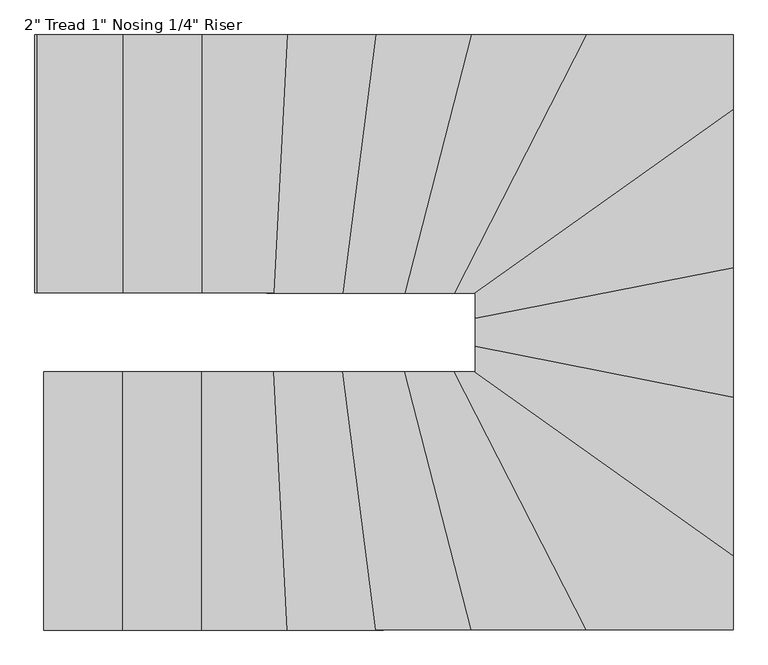
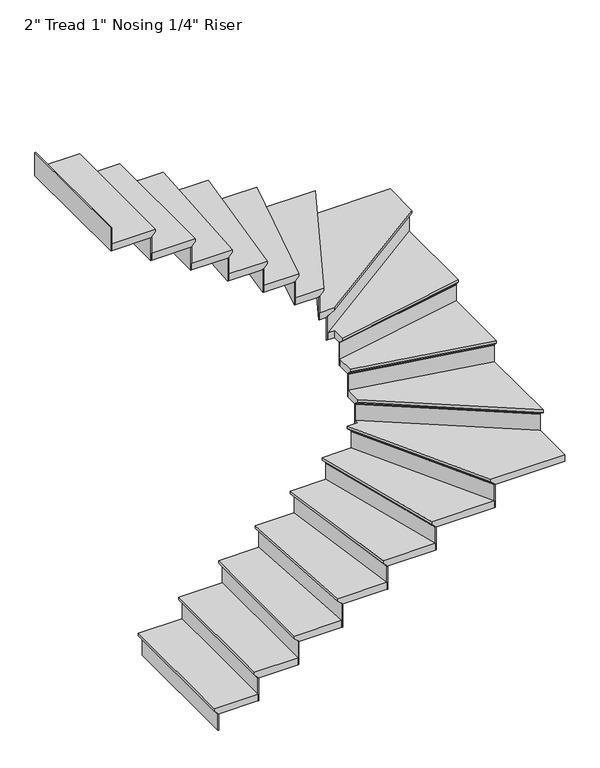
"""IFC4 building model written with IfcOpenShell, lengths in millimetres: stair flight geometry."""

from ifc_helpers import new_model, si_unit, origin, place, context, project, spatial, faceted_brep, source, transform, mapped, element, save


def stair_flight_09daeeff(model_context):
    return source(origin(), model_context, "Body", "Brep", [
        faceted_brep([(531.7538115, -7565.2090409, 16152.2833333), (531.7538115, -7565.2090409, 16171.3333333), (531.7538115, -6650.8090409, 16171.3333333), (531.7538115, -6650.8090409, 16152.2833333), (557.1538115, -7565.2090409, 16126.8833333), (557.1538115, -6650.8090409, 16126.8833333), (836.5538115, -7565.2090409, 16171.3333333), (836.5538115, -6650.8090409, 16171.3333333), (557.1538115, -6650.8090409, 16120.5333333), (836.5538115, -6650.8090409, 16120.5333333), (836.5538115, -7565.2090409, 16120.5333333), (557.1538115, -7565.2090409, 16120.5333333)], [[[0, 1, 2, 3]], [[4, 0, 3, 5]], [[2, 1, 6, 7]], [[8, 9, 10, 11]], [[2, 7, 9, 8, 5, 3]], [[8, 11, 4, 5]], [[6, 1, 0, 4, 11, 10]], [[7, 6, 10, 9]]]),
        faceted_brep([(557.1538115, -7565.2090409, 16120.5333333), (557.1538115, -7565.2090409, 16002.0), (563.5038115, -7565.2090409, 16002.0), (563.5038115, -7565.2090409, 16120.5333333), (557.1538115, -6650.8090409, 16120.5333333), (563.5038115, -6650.8090409, 16120.5333333), (563.5038115, -6650.8090409, 16002.0), (557.1538115, -6650.8090409, 16002.0)], [[[0, 1, 2, 3]], [[4, 5, 6, 7]], [[1, 0, 4, 7]], [[2, 1, 7, 6]], [[3, 2, 6, 5]], [[0, 3, 5, 4]]]),
        faceted_brep([(836.5538115, -7565.2090409, 16289.8666667), (836.5538115, -7565.2090409, 16120.5333333), (842.9038115, -7565.2090409, 16120.5333333), (842.9038115, -7565.2090409, 16289.8666667), (836.5538115, -6650.8090409, 16289.8666667), (842.9038115, -6650.8090409, 16289.8666667), (842.9038115, -6650.8090409, 16120.5333333), (836.5538115, -6650.8090409, 16120.5333333)], [[[0, 1, 2, 3]], [[4, 5, 6, 7]], [[1, 0, 4, 7]], [[2, 1, 7, 6]], [[3, 2, 6, 5]], [[0, 3, 5, 4]]]),
        faceted_brep([(811.1538115, -6650.8090409, 16340.6666667), (811.1538115, -7565.2090409, 16340.6666667), (1115.9538115, -7565.2090409, 16340.6666667), (1115.9538115, -6650.8090409, 16340.6666667), (836.5538115, -6650.8090409, 16289.8666667), (1115.9538115, -6650.8090409, 16289.8666667), (1115.9538115, -7565.2090409, 16289.8666667), (836.5538115, -7565.2090409, 16289.8666667), (836.5538115, -6650.8090409, 16296.2166667), (811.1538115, -6650.8090409, 16321.6166667), (836.5538115, -7565.2090409, 16296.2166667), (811.1538115, -7565.2090409, 16321.6166667)], [[[0, 1, 2, 3]], [[4, 5, 6, 7]], [[0, 3, 5, 4, 8, 9]], [[4, 7, 10, 8]], [[2, 1, 11, 10, 7, 6]], [[3, 2, 6, 5]], [[11, 1, 0, 9]], [[10, 11, 9, 8]]]),
        faceted_brep([(1115.9538115, -7565.2090409, 16459.2), (1115.9538115, -7565.2090409, 16289.8666667), (1122.3038115, -7565.2090409, 16289.8666667), (1122.3038115, -7565.2090409, 16459.2), (1115.9538115, -6650.8090409, 16459.2), (1122.3038115, -6650.8090409, 16459.2), (1122.3038115, -6650.8090409, 16289.8666667), (1115.9538115, -6650.8090409, 16289.8666667)], [[[0, 1, 2, 3]], [[4, 5, 6, 7]], [[1, 0, 4, 7]], [[2, 1, 7, 6]], [[3, 2, 6, 5]], [[0, 3, 5, 4]]]),
        faceted_brep([(1090.5538115, -6650.8090409, 16510.0), (1090.5538115, -7565.2090409, 16510.0), (1419.1552434, -7565.2090409, 16510.0), (1371.620973, -6650.8090409, 16510.0), (1115.9538115, -6650.8090409, 16459.2), (1371.620973, -6650.8090409, 16459.2), (1419.1552434, -7565.2090409, 16459.2), (1115.9538115, -7565.2090409, 16459.2), (1115.9538115, -6650.8090409, 16465.55), (1090.5538115, -6650.8090409, 16490.95), (1115.9538115, -7565.2090409, 16465.55), (1090.5538115, -7565.2090409, 16490.95)], [[[0, 1, 2, 3]], [[4, 5, 6, 7]], [[0, 3, 5, 4, 8, 9]], [[4, 7, 10, 8]], [[2, 1, 11, 10, 7, 6]], [[3, 2, 6, 5]], [[11, 1, 0, 9]], [[10, 11, 9, 8]]]),
        faceted_brep([(1419.1552434, -7565.2090409, 16628.5333333), (1419.1552434, -7565.2090409, 16459.2), (1425.5138176, -7565.2090409, 16459.2), (1425.5138176, -7565.2090409, 16628.5333333), (1371.620973, -6650.8090409, 16628.5333333), (1377.9795471, -6650.8090409, 16628.5333333), (1377.9795471, -6650.8090409, 16459.2), (1371.620973, -6650.8090409, 16459.2)], [[[0, 1, 2, 3]], [[4, 5, 6, 7]], [[1, 0, 4, 7]], [[2, 1, 7, 6]], [[3, 2, 6, 5]], [[0, 3, 5, 4]]]),
        faceted_brep([(1346.1866763, -6650.8090409, 16679.3333333), (1393.7209467, -7565.2090409, 16679.3333333), (1734.1437245, -7565.2090409, 16679.3333333), (1615.7876728, -6650.8090409, 16679.3333333), (1371.620973, -6650.8090409, 16628.5333333), (1615.7876728, -6650.8090409, 16628.5333333), (1734.1437245, -7565.2090409, 16628.5333333), (1419.1552434, -7565.2090409, 16628.5333333), (1371.620973, -6650.8090409, 16634.8833333), (1346.1866763, -6650.8090409, 16660.2833333), (1419.1552434, -7565.2090409, 16634.8833333), (1393.7209467, -7565.2090409, 16660.2833333)], [[[0, 1, 2, 3]], [[4, 5, 6, 7]], [[0, 3, 5, 4, 8, 9]], [[4, 7, 10, 8]], [[2, 1, 11, 10, 7, 6]], [[3, 2, 6, 5]], [[11, 1, 0, 9]], [[10, 11, 9, 8]]]),
        faceted_brep([(1734.1437245, -7565.2090409, 16797.8666667), (1734.1437245, -7565.2090409, 16628.5333333), (1740.5466962, -7565.2090409, 16628.5333333), (1740.5466962, -7565.2090409, 16797.8666667), (1615.7876728, -6650.8090409, 16797.8666667), (1622.1906446, -6650.8090409, 16797.8666667), (1622.1906446, -6650.8090409, 16628.5333333), (1615.7876728, -6650.8090409, 16628.5333333)], [[[0, 1, 2, 3]], [[4, 5, 6, 7]], [[1, 0, 4, 7]], [[2, 1, 7, 6]], [[3, 2, 6, 5]], [[0, 3, 5, 4]]]),
        faceted_brep([(1590.1757857, -6650.8090409, 16848.6666667), (1708.5318374, -7565.2090409, 16848.6666667), (2072.5453427, -7565.2090409, 16848.6666667), (1837.4148953, -6650.8090409, 16848.6666667), (1615.7876728, -6650.8090409, 16797.8666667), (1837.4148953, -6650.8090409, 16797.8666667), (2072.5453427, -7565.2090409, 16797.8666667), (1734.1437245, -7565.2090409, 16797.8666667), (1615.7876728, -6650.8090409, 16804.2166667), (1590.1757857, -6650.8090409, 16829.6166667), (1734.1437245, -7565.2090409, 16804.2166667), (1708.5318374, -7565.2090409, 16829.6166667)], [[[0, 1, 2, 3]], [[4, 5, 6, 7]], [[0, 3, 5, 4, 8, 9]], [[4, 7, 10, 8]], [[2, 1, 11, 10, 7, 6]], [[3, 2, 6, 5]], [[11, 1, 0, 9]], [[10, 11, 9, 8]]]),
        faceted_brep([(2072.5453427, -7565.2090409, 16967.2), (2072.5453427, -7565.2090409, 16797.8666667), (2079.1019196, -7565.2090409, 16797.8666667), (2079.1019196, -7565.2090409, 16967.2), (1837.4148953, -6650.8090409, 16967.2), (1843.9714722, -6650.8090409, 16967.2), (1843.9714722, -6650.8090409, 16797.8666667), (1837.4148953, -6650.8090409, 16797.8666667)], [[[0, 1, 2, 3]], [[4, 5, 6, 7]], [[1, 0, 4, 7]], [[2, 1, 7, 6]], [[3, 2, 6, 5]], [[0, 3, 5, 4]]]),
        faceted_brep([(1811.1885878, -6650.8090409, 17018.0), (2046.3190352, -7565.2090409, 17018.0), (2482.5861527, -7565.2090409, 17018.0), (2013.7615314, -6650.8090409, 17018.0), (1837.4148953, -6650.8090409, 16967.2), (2013.7615314, -6650.8090409, 16967.2), (2482.5861527, -7565.2090409, 16967.2), (2072.5453427, -7565.2090409, 16967.2), (1837.4148953, -6650.8090409, 16973.55), (1811.1885878, -6650.8090409, 16998.95), (2072.5453427, -7565.2090409, 16973.55), (2046.3190352, -7565.2090409, 16998.95)], [[[0, 1, 2, 3]], [[4, 5, 6, 7]], [[0, 3, 5, 4, 8, 9]], [[4, 7, 10, 8]], [[2, 1, 11, 10, 7, 6]], [[3, 2, 6, 5]], [[11, 1, 0, 9]], [[10, 11, 9, 8]]]),
        faceted_brep([(2482.5861527, -7565.2090409, 17136.5333333), (2482.5861527, -7565.2090409, 16967.2), (2489.7221358, -7565.2090409, 16967.2), (2489.7221358, -7565.2090409, 17136.5333333), (2013.7615314, -6650.8090409, 17136.5333333), (2020.8975145, -6650.8090409, 17136.5333333), (2020.8975145, -6650.8090409, 16967.2), (2013.7615314, -6650.8090409, 16967.2)], [[[0, 1, 2, 3]], [[4, 5, 6, 7]], [[1, 0, 4, 7]], [[2, 1, 7, 6]], [[3, 2, 6, 5]], [[0, 3, 5, 4]]]),
        faceted_brep([(2059.4855034, -6621.253958, 17187.3333333), (2059.4855034, -6650.8090409, 17187.3333333), (1985.2175988, -6650.8090409, 17187.3333333), (2454.0422202, -7565.2090409, 17187.3333333), (2973.8855034, -7565.2090409, 17187.3333333), (2973.8855034, -7271.5279072, 17187.3333333), (2059.4855034, -6650.8090409, 17136.5333333), (2059.4855034, -6621.253958, 17136.5333333), (2973.8855034, -7271.5279072, 17136.5333333), (2973.8855034, -7565.2090409, 17136.5333333), (2482.5861527, -7565.2090409, 17136.5333333), (2013.7615314, -6650.8090409, 17136.5333333), (2013.7615314, -6650.8090409, 17142.8833333), (1985.2175988, -6650.8090409, 17168.2833333), (2482.5861527, -7565.2090409, 17142.8833333), (2454.0422202, -7565.2090409, 17168.2833333)], [[[0, 1, 2, 3, 4, 5]], [[6, 7, 8, 9, 10, 11]], [[1, 0, 7, 6]], [[2, 1, 6, 11, 12, 13]], [[11, 10, 14, 12]], [[4, 3, 15, 14, 10, 9]], [[5, 4, 9, 8]], [[0, 5, 8, 7]], [[15, 3, 2, 13]], [[14, 15, 13, 12]]]),
        faceted_brep([(2973.8855034, -7271.5279072, 17305.8666667), (2973.8855034, -7271.5279072, 17136.5333333), (2973.8855034, -7263.7359324, 17136.5333333), (2973.8855034, -7263.7359324, 17305.8666667), (2059.4855034, -6621.253958, 17305.8666667), (2059.4855034, -6613.4619832, 17305.8666667), (2059.4855034, -6613.4619832, 17136.5333333), (2059.4855034, -6621.253958, 17136.5333333)], [[[0, 1, 2, 3]], [[4, 5, 6, 7]], [[1, 0, 4, 7]], [[2, 1, 7, 6]], [[3, 2, 6, 5]], [[0, 3, 5, 4]]]),
        faceted_brep([(2059.4855034, -6652.4218572, 17356.6666667), (2973.8855034, -7302.6958063, 17356.6666667), (2973.8855034, -6715.0407273, 17356.6666667), (2059.4855034, -6534.7998709, 17356.6666667), (2059.4855034, -6621.253958, 17305.8666667), (2059.4855034, -6534.7998709, 17305.8666667), (2973.8855034, -6715.0407273, 17305.8666667), (2973.8855034, -7271.5279072, 17305.8666667), (2059.4855034, -6621.253958, 17312.2166667), (2059.4855034, -6652.4218572, 17337.6166667), (2973.8855034, -7271.5279072, 17312.2166667), (2973.8855034, -7302.6958063, 17337.6166667)], [[[0, 1, 2, 3]], [[4, 5, 6, 7]], [[0, 3, 5, 4, 8, 9]], [[4, 7, 10, 8]], [[3, 2, 6, 5]], [[11, 1, 0, 9]], [[10, 11, 9, 8]], [[2, 1, 11, 10, 7, 6]]]),
        faceted_brep([(2973.8855034, -6715.0407273, 17475.2), (2973.8855034, -6715.0407273, 17305.8666667), (2973.8855034, -6708.5685418, 17305.8666667), (2973.8855034, -6708.5685418, 17475.2), (2059.4855034, -6534.7998709, 17475.2), (2059.4855034, -6528.3276855, 17475.2), (2059.4855034, -6528.3276855, 17305.8666667), (2059.4855034, -6534.7998709, 17305.8666667)], [[[0, 1, 2, 3]], [[4, 5, 6, 7]], [[1, 0, 4, 7]], [[2, 1, 7, 6]], [[3, 2, 6, 5]], [[0, 3, 5, 4]]]),
        faceted_brep([(2059.4855034, -6560.6886127, 17526.0), (2973.8855034, -6740.929469, 17526.0), (2973.8855034, -6255.3998709, 17526.0), (2059.4855034, -6435.6407273, 17526.0), (2059.4855034, -6534.7998709, 17475.2), (2059.4855034, -6435.6407273, 17475.2), (2973.8855034, -6255.3998709, 17475.2), (2973.8855034, -6715.0407273, 17475.2), (2059.4855034, -6534.7998709, 17481.55), (2059.4855034, -6560.6886127, 17506.95), (2973.8855034, -6715.0407273, 17481.55), (2973.8855034, -6740.929469, 17506.95)], [[[0, 1, 2, 3]], [[4, 5, 6, 7]], [[0, 3, 5, 4, 8, 9]], [[4, 7, 10, 8]], [[2, 1, 11, 10, 7, 6]], [[3, 2, 6, 5]], [[11, 1, 0, 9]], [[10, 11, 9, 8]]]),
        faceted_brep([(2973.8855034, -6255.3998709, 17644.5333333), (2973.8855034, -6255.3998709, 17475.2), (2973.8855034, -6248.9276855, 17475.2), (2973.8855034, -6248.9276855, 17644.5333333), (2059.4855034, -6435.6407273, 17644.5333333), (2059.4855034, -6429.1685418, 17644.5333333), (2059.4855034, -6429.1685418, 17475.2), (2059.4855034, -6435.6407273, 17475.2)], [[[0, 1, 2, 3]], [[4, 5, 6, 7]], [[1, 0, 4, 7]], [[2, 1, 7, 6]], [[3, 2, 6, 5]], [[0, 3, 5, 4]]]),
        faceted_brep([(2013.3900289, -6371.4090409, 17695.3333333), (2059.4855034, -6371.4090409, 17695.3333333), (2059.4855034, -6461.529469, 17695.3333333), (2973.8855034, -6281.2886127, 17695.3333333), (2973.8855034, -5688.3543762, 17695.3333333), (2059.4855034, -6371.4090409, 17644.5333333), (2013.3900289, -6371.4090409, 17644.5333333), (2973.8855034, -5688.3543762, 17644.5333333), (2973.8855034, -6255.3998709, 17644.5333333), (2059.4855034, -6435.6407273, 17644.5333333), (2973.8855034, -6255.3998709, 17650.8833333), (2059.4855034, -6435.6407273, 17650.8833333), (2973.8855034, -6281.2886127, 17676.2833333), (2059.4855034, -6461.529469, 17676.2833333)], [[[0, 1, 2, 3, 4]], [[5, 6, 7, 8, 9]], [[1, 0, 6, 5]], [[9, 8, 10, 11]], [[4, 3, 12, 10, 8, 7]], [[0, 4, 7, 6]], [[12, 3, 2, 13]], [[10, 12, 13, 11]], [[2, 1, 5, 9, 11, 13]]]),
        faceted_brep([(2973.8855034, -5688.3543762, 17813.8666667), (2973.8855034, -5688.3543762, 17644.5333333), (2973.8855034, -5680.5624014, 17644.5333333), (2973.8855034, -5680.5624014, 17813.8666667), (2013.3900289, -6371.4090409, 17813.8666667), (2002.4331364, -6371.4090409, 17813.8666667), (2002.4331364, -6371.4090409, 17644.5333333), (2013.3900289, -6371.4090409, 17644.5333333)], [[[0, 1, 2, 3]], [[4, 5, 6, 7]], [[1, 0, 4, 7]], [[2, 1, 7, 6]], [[3, 2, 6, 5]], [[0, 3, 5, 4]]]),
        faceted_brep([(2057.2175988, -6371.4090409, 17864.6666667), (2973.8855034, -5719.5222754, 17864.6666667), (2973.8855034, -5457.0090409, 17864.6666667), (2425.4982876, -5457.0090409, 17864.6666667), (1956.6736663, -6371.4090409, 17864.6666667), (2013.3900289, -6371.4090409, 17813.8666667), (1956.6736663, -6371.4090409, 17813.8666667), (2425.4982876, -5457.0090409, 17813.8666667), (2973.8855034, -5457.0090409, 17813.8666667), (2973.8855034, -5688.3543762, 17813.8666667), (2013.3900289, -6371.4090409, 17820.2166667), (2057.2175988, -6371.4090409, 17845.6166667), (2973.8855034, -5688.3543762, 17820.2166667), (2973.8855034, -5719.5222754, 17845.6166667)], [[[0, 1, 2, 3, 4]], [[5, 6, 7, 8, 9]], [[0, 4, 6, 5, 10, 11]], [[5, 9, 12, 10]], [[2, 1, 13, 12, 9, 8]], [[4, 3, 7, 6]], [[13, 1, 0, 11]], [[12, 13, 11, 10]], [[3, 2, 8, 7]]]),
        faceted_brep([(2425.4982876, -5457.0090409, 17983.2), (2425.4982876, -5457.0090409, 17813.8666667), (2418.3623045, -5457.0090409, 17813.8666667), (2418.3623045, -5457.0090409, 17983.2), (1956.6736663, -6371.4090409, 17983.2), (1949.5376832, -6371.4090409, 17983.2), (1949.5376832, -6371.4090409, 17813.8666667), (1956.6736663, -6371.4090409, 17813.8666667)], [[[0, 1, 2, 3]], [[4, 5, 6, 7]], [[1, 0, 4, 7]], [[2, 1, 7, 6]], [[3, 2, 6, 5]], [[0, 3, 5, 4]]]),
        faceted_brep([(1985.2175988, -6371.4090409, 18034.0), (2454.0422202, -5457.0090409, 18034.0), (2020.0927278, -5457.0090409, 18034.0), (1784.9622804, -6371.4090409, 18034.0), (1956.6736663, -6371.4090409, 17983.2), (1784.9622804, -6371.4090409, 17983.2), (2020.0927278, -5457.0090409, 17983.2), (2425.4982876, -5457.0090409, 17983.2), (1956.6736663, -6371.4090409, 17989.55), (1985.2175988, -6371.4090409, 18014.95), (2425.4982876, -5457.0090409, 17989.55), (2454.0422202, -5457.0090409, 18014.95)], [[[0, 1, 2, 3]], [[4, 5, 6, 7]], [[0, 3, 5, 4, 8, 9]], [[4, 7, 10, 8]], [[2, 1, 11, 10, 7, 6]], [[3, 2, 6, 5]], [[11, 1, 0, 9]], [[10, 11, 9, 8]]]),
        faceted_brep([(2020.0927278, -5457.0090409, 18152.5333333), (2020.0927278, -5457.0090409, 17983.2), (2013.5361509, -5457.0090409, 17983.2), (2013.5361509, -5457.0090409, 18152.5333333), (1784.9622804, -6371.4090409, 18152.5333333), (1778.4057035, -6371.4090409, 18152.5333333), (1778.4057035, -6371.4090409, 17983.2), (1784.9622804, -6371.4090409, 17983.2)], [[[0, 1, 2, 3]], [[4, 5, 6, 7]], [[1, 0, 4, 7]], [[2, 1, 7, 6]], [[3, 2, 6, 5]], [[0, 3, 5, 4]]]),
        faceted_brep([(1811.1885878, -6371.4090409, 18203.3333333), (2046.3190352, -5457.0090409, 18203.3333333), (1682.9199502, -5457.0090409, 18203.3333333), (1564.5638986, -6371.4090409, 18203.3333333), (1784.9622804, -6371.4090409, 18152.5333333), (1564.5638986, -6371.4090409, 18152.5333333), (1682.9199502, -5457.0090409, 18152.5333333), (2020.0927278, -5457.0090409, 18152.5333333), (1784.9622804, -6371.4090409, 18158.8833333), (1811.1885878, -6371.4090409, 18184.2833333), (2020.0927278, -5457.0090409, 18158.8833333), (2046.3190352, -5457.0090409, 18184.2833333)], [[[0, 1, 2, 3]], [[4, 5, 6, 7]], [[0, 3, 5, 4, 8, 9]], [[4, 7, 10, 8]], [[2, 1, 11, 10, 7, 6]], [[3, 2, 6, 5]], [[11, 1, 0, 9]], [[10, 11, 9, 8]]]),
        faceted_brep([(1682.9199502, -5457.0090409, 18321.8666667), (1682.9199502, -5457.0090409, 18152.5333333), (1676.5169785, -5457.0090409, 18152.5333333), (1676.5169785, -5457.0090409, 18321.8666667), (1564.5638986, -6371.4090409, 18321.8666667), (1558.1609268, -6371.4090409, 18321.8666667), (1558.1609268, -6371.4090409, 18152.5333333), (1564.5638986, -6371.4090409, 18152.5333333)], [[[0, 1, 2, 3]], [[4, 5, 6, 7]], [[1, 0, 4, 7]], [[2, 1, 7, 6]], [[3, 2, 6, 5]], [[0, 3, 5, 4]]]),
        faceted_brep([(1590.1757857, -6371.4090409, 18372.6666667), (1708.5318374, -5457.0090409, 18372.6666667), (1368.2866501, -5457.0090409, 18372.6666667), (1320.7523797, -6371.4090409, 18372.6666667), (1564.5638986, -6371.4090409, 18321.8666667), (1320.7523797, -6371.4090409, 18321.8666667), (1368.2866501, -5457.0090409, 18321.8666667), (1682.9199502, -5457.0090409, 18321.8666667), (1564.5638986, -6371.4090409, 18328.2166667), (1590.1757857, -6371.4090409, 18353.6166667), (1682.9199502, -5457.0090409, 18328.2166667), (1708.5318374, -5457.0090409, 18353.6166667)], [[[0, 1, 2, 3]], [[4, 5, 6, 7]], [[0, 3, 5, 4, 8, 9]], [[4, 7, 10, 8]], [[2, 1, 11, 10, 7, 6]], [[3, 2, 6, 5]], [[11, 1, 0, 9]], [[10, 11, 9, 8]]]),
        faceted_brep([(1368.2866501, -5457.0090409, 18491.2), (1368.2866501, -5457.0090409, 18321.8666667), (1361.9280759, -5457.0090409, 18321.8666667), (1361.9280759, -5457.0090409, 18491.2), (1320.7523797, -6371.4090409, 18491.2), (1314.3938055, -6371.4090409, 18491.2), (1314.3938055, -6371.4090409, 18321.8666667), (1320.7523797, -6371.4090409, 18321.8666667)], [[[0, 1, 2, 3]], [[4, 5, 6, 7]], [[1, 0, 4, 7]], [[2, 1, 7, 6]], [[3, 2, 6, 5]], [[0, 3, 5, 4]]]),
        faceted_brep([(1346.1866763, -6371.4090409, 18542.0), (1393.7209467, -5457.0090409, 18542.0), (1065.1538115, -5457.0090409, 18542.0), (1065.1538115, -6371.4090409, 18542.0), (1320.7523797, -6371.4090409, 18491.2), (1065.1538115, -6371.4090409, 18491.2), (1065.1538115, -5457.0090409, 18491.2), (1368.2866501, -5457.0090409, 18491.2), (1320.7523797, -6371.4090409, 18497.55), (1346.1866763, -6371.4090409, 18522.95), (1368.2866501, -5457.0090409, 18497.55), (1393.7209467, -5457.0090409, 18522.95)], [[[0, 1, 2, 3]], [[4, 5, 6, 7]], [[0, 3, 5, 4, 8, 9]], [[4, 7, 10, 8]], [[2, 1, 11, 10, 7, 6]], [[3, 2, 6, 5]], [[11, 1, 0, 9]], [[10, 11, 9, 8]]]),
        faceted_brep([(1065.1538115, -5457.0090409, 18660.5333333), (1065.1538115, -5457.0090409, 18491.2), (1058.8038115, -5457.0090409, 18491.2), (1058.8038115, -5457.0090409, 18660.5333333), (1065.1538115, -6371.4090409, 18660.5333333), (1058.8038115, -6371.4090409, 18660.5333333), (1058.8038115, -6371.4090409, 18491.2), (1065.1538115, -6371.4090409, 18491.2)], [[[0, 1, 2, 3]], [[4, 5, 6, 7]], [[1, 0, 4, 7]], [[2, 1, 7, 6]], [[3, 2, 6, 5]], [[0, 3, 5, 4]]]),
        faceted_brep([(1090.5538115, -6371.4090409, 18711.3333333), (1090.5538115, -5457.0090409, 18711.3333333), (785.7538115, -5457.0090409, 18711.3333333), (785.7538115, -6371.4090409, 18711.3333333), (1065.1538115, -6371.4090409, 18660.5333333), (785.7538115, -6371.4090409, 18660.5333333), (785.7538115, -5457.0090409, 18660.5333333), (1065.1538115, -5457.0090409, 18660.5333333), (1065.1538115, -6371.4090409, 18666.8833333), (1090.5538115, -6371.4090409, 18692.2833333), (1065.1538115, -5457.0090409, 18666.8833333), (1090.5538115, -5457.0090409, 18692.2833333)], [[[0, 1, 2, 3]], [[4, 5, 6, 7]], [[0, 3, 5, 4, 8, 9]], [[4, 7, 10, 8]], [[2, 1, 11, 10, 7, 6]], [[3, 2, 6, 5]], [[11, 1, 0, 9]], [[10, 11, 9, 8]]]),
        faceted_brep([(785.7538115, -5457.0090409, 18829.8666667), (785.7538115, -5457.0090409, 18660.5333333), (779.4038115, -5457.0090409, 18660.5333333), (779.4038115, -5457.0090409, 18829.8666667), (785.7538115, -6371.4090409, 18829.8666667), (779.4038115, -6371.4090409, 18829.8666667), (779.4038115, -6371.4090409, 18660.5333333), (785.7538115, -6371.4090409, 18660.5333333)], [[[0, 1, 2, 3]], [[4, 5, 6, 7]], [[1, 0, 4, 7]], [[2, 1, 7, 6]], [[3, 2, 6, 5]], [[0, 3, 5, 4]]]),
        faceted_brep([(506.3538115, -5457.0090409, 18999.2), (506.3538115, -5457.0090409, 18829.8666667), (500.0038115, -5457.0090409, 18829.8666667), (500.0038115, -5457.0090409, 18999.2), (506.3538115, -6371.4090409, 18999.2), (500.0038115, -6371.4090409, 18999.2), (500.0038115, -6371.4090409, 18829.8666667), (506.3538115, -6371.4090409, 18829.8666667)], [[[0, 1, 2, 3]], [[4, 5, 6, 7]], [[1, 0, 4, 7]], [[2, 1, 7, 6]], [[3, 2, 6, 5]], [[0, 3, 5, 4]]]),
        faceted_brep([(811.1538115, -6371.4090409, 18880.6666667), (811.1538115, -5457.0090409, 18880.6666667), (506.3538115, -5457.0090409, 18880.6666667), (506.3538115, -6371.4090409, 18880.6666667), (785.7538115, -6371.4090409, 18829.8666667), (506.3538115, -6371.4090409, 18829.8666667), (506.3538115, -5457.0090409, 18829.8666667), (785.7538115, -5457.0090409, 18829.8666667), (785.7538115, -6371.4090409, 18836.2166667), (811.1538115, -6371.4090409, 18861.6166667), (785.7538115, -5457.0090409, 18836.2166667), (811.1538115, -5457.0090409, 18861.6166667)], [[[0, 1, 2, 3]], [[4, 5, 6, 7]], [[0, 3, 5, 4, 8, 9]], [[4, 7, 10, 8]], [[2, 1, 11, 10, 7, 6]], [[3, 2, 6, 5]], [[11, 1, 0, 9]], [[10, 11, 9, 8]]]),
    ])


if __name__ == "__main__":
    model = new_model("IFC4")
    model_context = context("Model", 3, world=origin())
    ifc_project = project(units=[si_unit("LENGTHUNIT", "METRE", prefix="MILLI")], contexts=[model_context])
    site = spatial("IfcSite", under=ifc_project)
    building = spatial("IfcBuilding", under=site)
    placement = place(None, origin())
    stair_flight_shape = stair_flight_09daeeff(model_context)
    element("IfcStairFlight", 1, ObjectType="2\" Tread 1\" Nosing 1/4\" Riser", at=placement, inside=building, context=model_context, shape_type="MappedRepresentation", body=[
        mapped(stair_flight_shape, transform((0.0, 0.0, 0.0), x_axis=(1.0, 0.0, 0.0), y_axis=(0.0, 1.0, 0.0), z_axis=(0.0, 0.0, 1.0))),
    ])
    save(model, "model.ifc")
